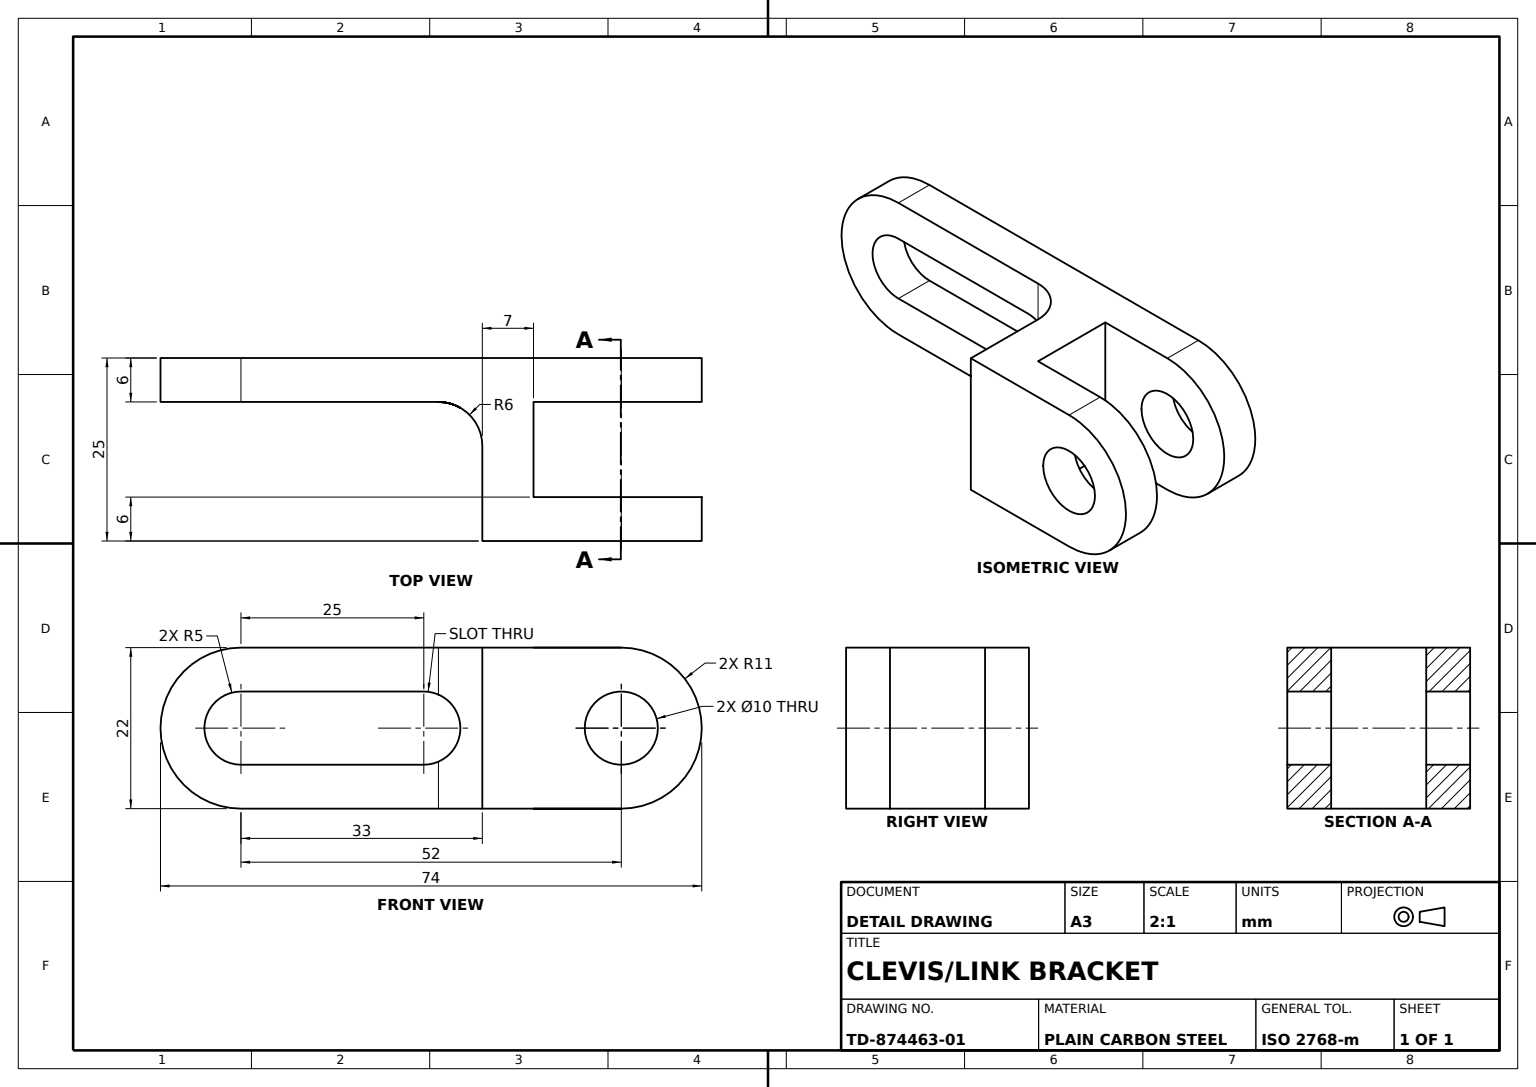
SolidWorks part; units mm, degrees
material "Plain Carbon Steel"
ref_plane "Front Plane" through (0, 0, 0) normal (0, 0, 1) x (1, 0, 0)
ref_plane "Top Plane" through (0, 0, 0) normal (0, 1, 0) x (1, 0, 0)
ref_plane "Right Plane" through (0, 0, 0) normal (1, 0, 0) x (0, 0, -1)
sketch "Base Block Sketch" plane through (0, 0, 0) normal (0, 0, 1) x (1, 0, 0)
  line L1 (0, 11) -> (52, 11)
  line L3 (52, -11) -> (0, -11)
  arc A0 (0, 11) -> (0, -11) centre (0, 0) ccw
  arc A1 (52, -11) -> (52, 11) centre (52, 0) ccw
  dimension "D1" = 22
  dimension "D2" = 22
  dimension "D3" = 11
  dimension "D4" = 52
extrude "Base Block 22x22" add sketch "Base Block Sketch" along normal blind 6
sketch "Square Cutout Sketch" plane through (0, 0, 6) normal (0, 0, 1) x (1, 0, 0)
  line L1 (0, 5) -> (25, 5)
  line L3 (25, -5) -> (0, -5)
  arc A0 (0, 5) -> (0, -5) centre (0, 0) ccw
  arc A1 (25, -5) -> (25, 5) centre (25, 0) ccw
  dimension "D1" = 10
  dimension "D2" = 10
  dimension "D3" = 5
  dimension "D4" = 25
extrude "Square Cutout 10x10" cut sketch "Square Cutout Sketch" against normal blind 6
sketch "Link Profile Sketch" plane through (0, -11, 0) normal (0, -1, 0) x (1, 0, 0)
  line L0 (27, 6) -> (33, 6)
  line L1 (0, 6) -> (52, 6) construction
  line L2 (33, 12) -> (33, 19)
  line L4 (33, 6) -> (40, 6)
  line L6 (33, 19) -> (33, 25)
  line L13 (0, 0) -> (52, 0) construction
  line L14 (33, 25) -> (52, 25)
  line L15 (40, 6) -> (40, 19)
  line L16 (40, 19) -> (52, 19)
  line L17 (52, 25) -> (52, 19)
  arc A0 (27, 6) -> (33, 12) centre (27, 12) ccw
  dimension "D2" = 12
  dimension "D1" = 25
  dimension "D3" = 27
  dimension "D4" = 7
  dimension "D5" = 7
  dimension "D6" = 12
  dimension "D7" = 33
extrude "Link Body" add sketch "Link Profile Sketch" against normal blind 22
sketch "Link Slot Sketch" plane through (0, 0, 6) normal (0, 0, -1) x (-1, 0, 0)
  line L0 (-27, 4.5826) -> (-27, -4.5826)
  arc A0 (-27, 4.5826) -> (-27, -4.5826) centre (-25, 0) ccw
  dimension "D1" = 10
extrude "Link Slot" cut sketch "Link Slot Sketch" against normal blind 22
sketch "End Tab Sketch" plane through (0, 0, 25) normal (0, 0, 1) x (1, 0, 0)
  line L0 (52, 11) -> (52, -11) construction
  line L1 (52, 11) -> (52, -11)
  arc A0 (52, -11) -> (52, 11) centre (52, 0) ccw
  dimension "D1" = 22
extrude "End Tab" add sketch "End Tab Sketch" against normal blind 6
sketch "Cross Hole Sketch" plane through (0, 0, 25) normal (0, 0, 1) x (1, 0, 0)
  circle A0 centre (52, 0) radius 5
  dimension "D1" = 10
  dimension "D2" = 10
extrude "Cross Hole Ø10" cut sketch "Cross Hole Sketch" against normal blind 25
